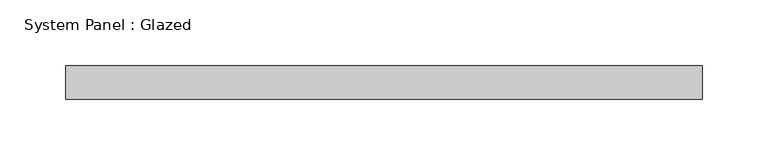
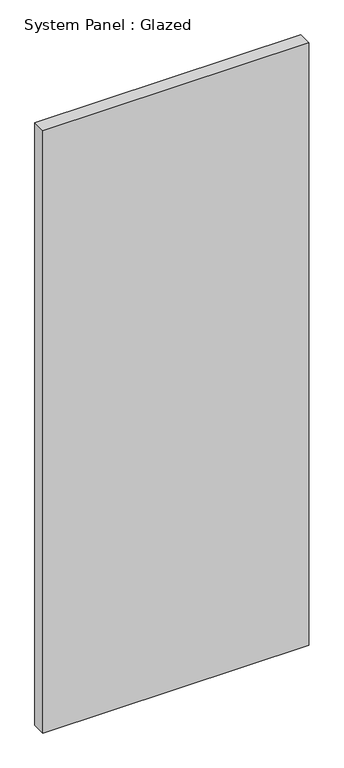
"""IFC4 building model written with IfcOpenShell, lengths in millimetres: plate geometry, System Panel : Glazed."""

from ifc_helpers import new_model, si_unit, origin, origin_with_axes, place, context, project, spatial, polyline, outline, extrude, source, transform, mapped, element, save


def system_panel_glazed_cd2dd794(model_context):
    return source(origin(), model_context, "Body", "SweptSolid", [
        extrude(outline(polyline([(241.3, 19.05), (-241.3, 19.05), (-241.3, 44.45), (241.3, 44.45), (241.3, 19.05)])), origin_with_axes(), (0.0, 0.0, 1.0), 1155.7),
    ])


if __name__ == "__main__":
    model = new_model("IFC4")
    model_context = context("Model", 3, world=origin())
    ifc_project = project(units=[si_unit("LENGTHUNIT", "METRE", prefix="MILLI")], contexts=[model_context])
    site = spatial("IfcSite", under=ifc_project)
    building = spatial("IfcBuilding", under=site)
    placement = place(None, origin())
    system_panel_glazed_shape = system_panel_glazed_cd2dd794(model_context)
    element("IfcPlate", 1, ObjectType="System Panel : Glazed", at=placement, inside=building, context=model_context, shape_type="MappedRepresentation", body=[
        mapped(system_panel_glazed_shape, transform((0.0, 0.0, 0.0), x_axis=(1.0, 0.0, 0.0), y_axis=(0.0, 1.0, 0.0), z_axis=(0.0, 0.0, 1.0))),
    ])
    save(model, "model.ifc")

# Revit data of these elements
# Type "System Panel : Glazed"
#   Construction Type Id = "GSP4R"
#   Analytic Construction = "1/8 in Pilkington single glazing"
#   Visual Light Transmittance = 0.9
#   Solar Heat Gain Coefficient = 0.86
#   Heat Transfer Coefficient (U) = 1.18115 BTU/(h·ft²·°F)
#   Define Thermal Properties by = 1
# Element 1 (IfcPlate, "System Panel : Glazed")
#   Materials on its faces: "Glass"
# Materials
#   "Glass": class "Glass", colour RGB 0 128 192, transparency 0.75, Description = "Soda Lime Glass", Cost = 0
